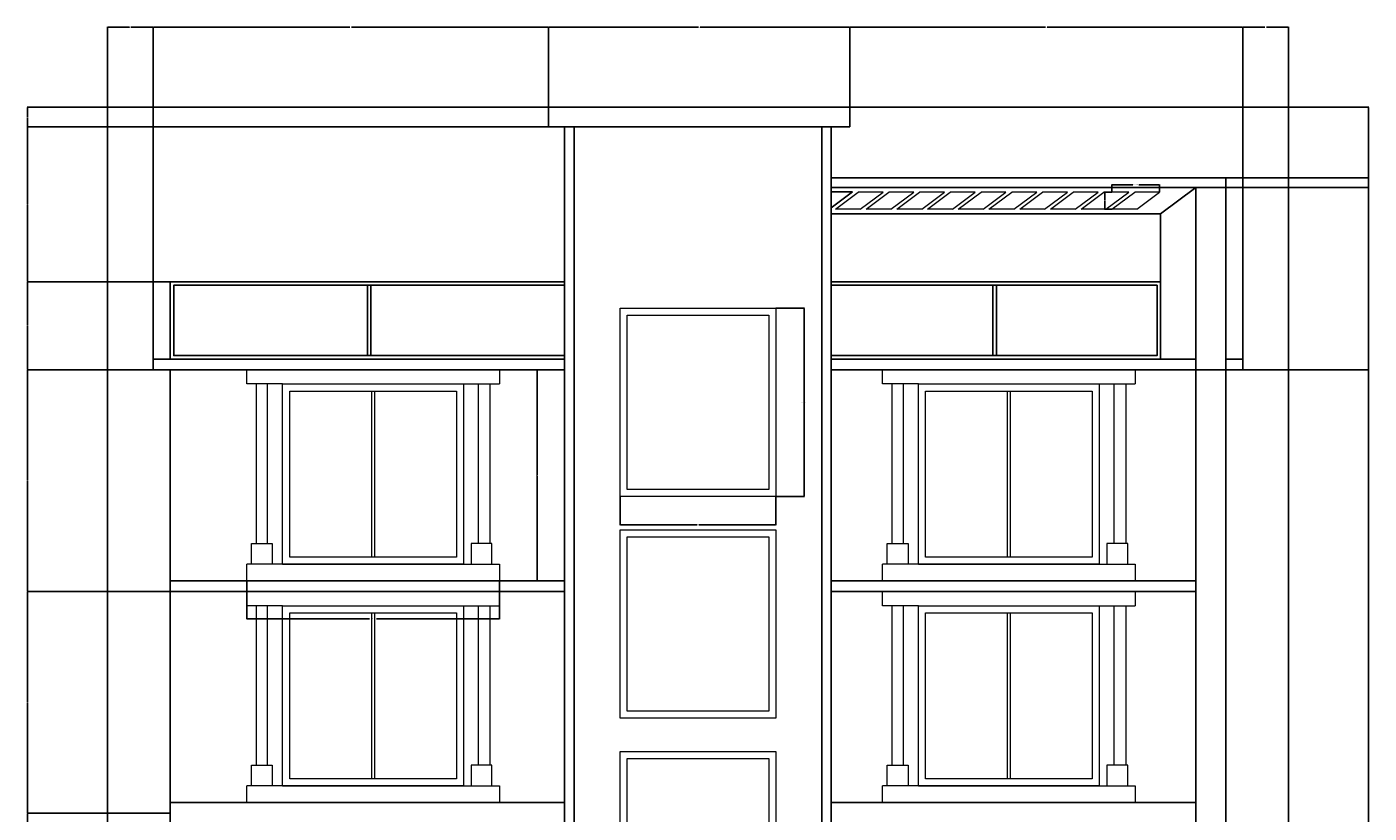
# Model space of a CAD drawing. Units: inches. Extents: x 3024 to 4744, y 1110 to 2100.
# Tile 29 of 29: x 3980 to 4744, y 1654 to 2100. Entities that reach past the tile are written whole.
import ezdxf

# ---------------------------------------------------------------- set-up
doc = ezdxf.new("R2010")
doc.units = ezdxf.units.IN
for name, color, linetype, lineweight in [('A-ANNO-DIMS', 2, 'Continuous', 18), ('A-ELEV', 7, 'Continuous', 25), ('A-GLAZ', 4, 'Continuous', 18), ('A-ROOF', 3, 'Continuous', 18)]:
    doc.layers.add(name, color=color, linetype=linetype, lineweight=lineweight)
doc.styles.get("Standard").update_dxf_attribs({"font": 'arial.ttf'})
doc.dimstyles.get("Standard").update_dxf_attribs({"dimtxt": 0.18, "dimasz": 0.18, "dimexe": 0.18, "dimexo": 0.0625, "dimgap": 0.09, "dimtad": 0, "dimtih": 1, "dimtoh": 1, "dimdec": 1, "dimzin": 0, "dimdsep": 46, "dimlunit": 3, "dimtxsty": 'Standard', "dimcen": 0.09, "dimadec": 0, "dimazin": 0, "dimtfac": 1, "dimtdec": 1, "dimtofl": 0, "dimtmove": 0, "dimatfit": 3, "dimfxl": 1, "dimtolj": 1, "dimtzin": 0, "dimarcsym": 0})

# ---------------------------------------------------------------- blocks, each defined once
blk = doc.blocks.new('WIN-BALCONY-B')
for p, q in [((4125.9, 1897.49), (4105.47, 1897.49)), ((4125.9, 1897.49), (4249.1, 1897.49)), ((4125.9, 1795.04), (4105.47, 1795.04)), ((4125.9, 1795.04), (4249.1, 1795.04))]:
    blk.add_line(p, q)
for points in [[(4105.47, 1897.49), (4105.47, 1905.61), (4249.1, 1905.61), (4249.1, 1897.49)], [(4249.1, 1795.04), (4249.1, 1785.61), (4105.47, 1785.61), (4105.47, 1795.04)]]:
    blk.add_lwpolyline(points)
for points in [[(4110.83, 1806.87), (4117.36, 1806.87), (4117.36, 1897.49), (4110.83, 1897.49)], [(4228.68, 1795.04), (4125.9, 1795.04), (4125.9, 1897.49), (4228.68, 1897.49)], [(4224.68, 1799.04), (4129.9, 1799.04), (4129.9, 1893.49), (4224.68, 1893.49)], [(4176.55, 1893.49), (4178.02, 1893.49), (4178.02, 1799.04), (4176.55, 1799.04)], [(4243.74, 1806.87), (4237.21, 1806.87), (4237.21, 1897.49), (4243.74, 1897.49)], [(4120.03, 1795.04), (4108.16, 1795.04), (4108.16, 1806.87), (4120.03, 1806.87)], [(4233.01, 1795.04), (4244.87, 1795.04), (4244.87, 1806.87), (4233.01, 1806.87)]]:
    blk.add_lwpolyline(points, close=True)
blk = doc.blocks.new('PERGOLA-RAFTER')
for p, q in [((13, 9.73), (0, 0)), ((13, 9.73), (27.14, 9.72)), ((27.14, 9.72), (14.16, 0.01)), ((0, 0), (14.16, 0.01))]:
    blk.add_line(p, q)
blk = doc.blocks.new('WIN-CENTRE-PLAIN')
for points in [[(4317.72, 1940.61), (4406.22, 1940.61), (4406.22, 1833.52), (4317.72, 1833.52)], [(4321.72, 1936.61), (4402.22, 1936.61), (4402.22, 1837.52), (4321.72, 1837.52)]]:
    blk.add_lwpolyline(points, close=True)
blk = doc.blocks.new('*D8')
at = {"layer": 'A-ANNO-DIMS', "color": 0, "lineweight": -2, "transparency": 16777216}
for p, q in [((4105.47, 1785.55), (4105.47, 1763.89)), ((4249.1, 1785.55), (4249.1, 1763.89)), ((4105.65, 1764.07), (4175.35, 1764.07)), ((4248.92, 1764.07), (4179.22, 1764.07))]:
    blk.add_line(p, q, dxfattribs=at)
at = {"layer": 'A-ANNO-DIMS', "color": 0, "transparency": 16777216}
for points in [[(4105.65, 1764.1), (4105.65, 1764.04), (4105.47, 1764.07)], [(4248.92, 1764.1), (4248.92, 1764.04), (4249.1, 1764.07)]]:
    blk.add_solid(points, dxfattribs=at)
at = {"layer": 'Defpoints', "color": 0, "transparency": 16777216}
for p in [(4105.47, 1785.61), (4249.1, 1785.61), (4249.1, 1764.07)]:
    blk.add_point(p, dxfattribs=at)
at = {"layer": 'A-ANNO-DIMS', "color": 0, "transparency": 16777216, "insert": (4177.29, 1764.07), "char_height": 0.18, "attachment_point": 5}
blk.add_mtext('\\A1;BALCONY WINDOW B 144 TYP.', dxfattribs=at)
blk = doc.blocks.new('*D9')
at = {"layer": 'A-ANNO-DIMS', "color": 0, "lineweight": -2, "transparency": 16777216}
for p, q in [((4249.17, 1905.61), (4270.83, 1905.61)), ((4270.65, 1905.43), (4270.65, 1845.79)), ((4270.65, 1785.79), (4270.65, 1845.43)), ((4249.17, 1785.61), (4270.83, 1785.61))]:
    blk.add_line(p, q, dxfattribs=at)
at = {"layer": 'A-ANNO-DIMS', "color": 0, "transparency": 16777216}
for points in [[(4270.62, 1905.43), (4270.68, 1905.43), (4270.65, 1905.61)], [(4270.62, 1785.79), (4270.68, 1785.79), (4270.65, 1785.61)]]:
    blk.add_solid(points, dxfattribs=at)
at = {"layer": 'Defpoints', "color": 0, "transparency": 16777216}
for p in [(4249.1, 1905.61), (4270.65, 1905.61), (4249.1, 1785.61)]:
    blk.add_point(p, dxfattribs=at)
at = {"layer": 'A-ANNO-DIMS', "color": 0, "transparency": 16777216, "insert": (4270.65, 1845.61), "char_height": 0.18, "attachment_point": 5}
blk.add_mtext('\\A1;120 TYP.', dxfattribs=at)
blk = doc.blocks.new('*D12')
at = {"layer": 'A-ANNO-DIMS', "color": 0, "lineweight": -2, "transparency": 16777216}
for p, q in [((4406.28, 1940.61), (4422.46, 1940.61)), ((4422.28, 1940.43), (4422.28, 1887.25)), ((4422.28, 1833.7), (4422.28, 1886.88)), ((4406.28, 1833.52), (4422.46, 1833.52))]:
    blk.add_line(p, q, dxfattribs=at)
at = {"layer": 'A-ANNO-DIMS', "color": 0, "transparency": 16777216}
for points in [[(4422.25, 1940.43), (4422.31, 1940.43), (4422.28, 1940.61)], [(4422.25, 1833.7), (4422.31, 1833.7), (4422.28, 1833.52)]]:
    blk.add_solid(points, dxfattribs=at)
at = {"layer": 'Defpoints', "color": 0, "transparency": 16777216}
for p in [(4406.22, 1940.61), (4422.28, 1940.61), (4406.22, 1833.52)]:
    blk.add_point(p, dxfattribs=at)
at = {"layer": 'A-ANNO-DIMS', "color": 0, "transparency": 16777216, "insert": (4422.28, 1887.07), "char_height": 0.18, "attachment_point": 5}
blk.add_mtext('\\A1;CENTRE WINDOW 107 TYP.', dxfattribs=at)
blk = doc.blocks.new('*D13')
at = {"layer": 'A-ANNO-DIMS', "color": 0, "lineweight": -2, "transparency": 16777216}
for p, q in [((4317.72, 1833.46), (4317.72, 1817.28)), ((4406.22, 1833.46), (4406.22, 1817.28)), ((4317.9, 1817.46), (4361.44, 1817.46)), ((4406.04, 1817.46), (4362.5, 1817.46))]:
    blk.add_line(p, q, dxfattribs=at)
at = {"layer": 'A-ANNO-DIMS', "color": 0, "transparency": 16777216}
for points in [[(4317.9, 1817.49), (4317.9, 1817.43), (4317.72, 1817.46)], [(4406.04, 1817.49), (4406.04, 1817.43), (4406.22, 1817.46)]]:
    blk.add_solid(points, dxfattribs=at)
at = {"layer": 'Defpoints', "color": 0, "transparency": 16777216}
for p in [(4317.72, 1833.52), (4406.22, 1833.52), (4406.22, 1817.46)]:
    blk.add_point(p, dxfattribs=at)
at = {"layer": 'A-ANNO-DIMS', "color": 0, "transparency": 16777216, "insert": (4361.97, 1817.46), "char_height": 0.18, "attachment_point": 5}
blk.add_mtext('\\A1;88 TYP.', dxfattribs=at)
blk = doc.blocks.new('*D14')
at = {"layer": 'A-ANNO-DIMS', "color": 0, "lineweight": -2, "transparency": 16777216}
for p, q in [((4597.25, 2006.58), (4597.25, 2010.77)), ((4597.43, 2010.59), (4609.12, 2010.58)), ((4624.21, 2010.58), (4612.53, 2010.58)), ((4624.39, 2006.57), (4624.39, 2010.76))]:
    blk.add_line(p, q, dxfattribs=at)
at = {"layer": 'A-ANNO-DIMS', "color": 0, "transparency": 16777216}
for points in [[(4597.43, 2010.62), (4597.43, 2010.56), (4597.25, 2010.59)], [(4624.21, 2010.61), (4624.21, 2010.55), (4624.39, 2010.58)]]:
    blk.add_solid(points, dxfattribs=at)
at = {"layer": 'Defpoints', "color": 0, "transparency": 16777216}
for p in [(4597.25, 2010.59), (4597.25, 2006.52), (4624.39, 2006.51)]:
    blk.add_point(p, dxfattribs=at)
at = {"layer": 'A-ANNO-DIMS', "color": 0, "transparency": 16777216, "insert": (4610.82, 2010.58), "char_height": 0.18, "attachment_point": 5}
blk.add_mtext('\\A1;PERGOLA RAFTER 27 TYP.', dxfattribs=at)
blk = doc.blocks.new('*D15')
at = {"layer": 'A-ANNO-DIMS', "color": 0, "lineweight": -2, "transparency": 16777216}
for p, q in [((4597.19, 2006.52), (4593, 2006.52)), ((4593.18, 2006.34), (4593.18, 2001.84)), ((4593.18, 1996.97), (4593.18, 2001.47)), ((4597.18, 1996.79), (4593, 1996.79))]:
    blk.add_line(p, q, dxfattribs=at)
at = {"layer": 'A-ANNO-DIMS', "color": 0, "transparency": 16777216}
for points in [[(4593.15, 2006.34), (4593.21, 2006.34), (4593.18, 2006.52)], [(4593.15, 1996.97), (4593.21, 1996.97), (4593.18, 1996.79)]]:
    blk.add_solid(points, dxfattribs=at)
at = {"layer": 'Defpoints', "color": 0, "transparency": 16777216}
for p in [(4597.25, 2006.52), (4593.18, 1996.79), (4597.25, 1996.79)]:
    blk.add_point(p, dxfattribs=at)
at = {"layer": 'A-ANNO-DIMS', "color": 0, "transparency": 16777216, "insert": (4593.18, 2001.65), "char_height": 0.18, "attachment_point": 5}
blk.add_mtext('\\A1;10 TYP.', dxfattribs=at)
blk = doc.blocks.new('*D30')
at = {"layer": 'A-ANNO-DIMS', "color": 0, "lineweight": -2, "transparency": 16777216}
for p, q in [((4026.29, 1241.5), (4026.29, 2100.44)), ((4026.47, 2100.26), (4038.86, 2100.26)), ((4052.03, 2100.26), (4039.65, 2100.26)), ((4052.21, 1911.67), (4052.21, 2100.44))]:
    blk.add_line(p, q, dxfattribs=at)
at = {"layer": 'A-ANNO-DIMS', "color": 0, "transparency": 16777216}
for points in [[(4026.47, 2100.29), (4026.47, 2100.23), (4026.29, 2100.26)], [(4052.03, 2100.29), (4052.03, 2100.23), (4052.21, 2100.26)]]:
    blk.add_solid(points, dxfattribs=at)
at = {"layer": 'Defpoints', "color": 0, "transparency": 16777216}
for p in [(4052.21, 2100.26), (4052.21, 1911.61), (4026.29, 1241.43)]:
    blk.add_point(p, dxfattribs=at)
at = {"layer": 'A-ANNO-DIMS', "color": 0, "transparency": 16777216, "insert": (4039.25, 2100.26), "char_height": 0.18, "attachment_point": 5}
blk.add_mtext('\\A1;25.92', dxfattribs=at)
blk = doc.blocks.new('*D31')
at = {"layer": 'A-ANNO-DIMS', "color": 0, "lineweight": -2, "transparency": 16777216}
for p, q in [((4052.21, 1911.67), (4052.21, 2100.44)), ((4052.39, 2100.26), (4164.17, 2100.26)), ((4276.88, 2100.26), (4165.11, 2100.26)), ((4277.06, 2054.82), (4277.06, 2100.44))]:
    blk.add_line(p, q, dxfattribs=at)
at = {"layer": 'A-ANNO-DIMS', "color": 0, "transparency": 16777216}
for points in [[(4052.39, 2100.29), (4052.39, 2100.23), (4052.21, 2100.26)], [(4276.88, 2100.29), (4276.88, 2100.23), (4277.06, 2100.26)]]:
    blk.add_solid(points, dxfattribs=at)
at = {"layer": 'Defpoints', "color": 0, "transparency": 16777216}
for p in [(4277.06, 2100.26), (4277.06, 2054.76), (4052.21, 1911.61)]:
    blk.add_point(p, dxfattribs=at)
at = {"layer": 'A-ANNO-DIMS', "color": 0, "transparency": 16777216, "insert": (4164.64, 2100.26), "char_height": 0.18, "attachment_point": 5}
blk.add_mtext('\\A1;224.85', dxfattribs=at)
blk = doc.blocks.new('*D32')
at = {"layer": 'A-ANNO-DIMS', "color": 0, "lineweight": -2, "transparency": 16777216}
for p, q in [((4277.06, 2054.82), (4277.06, 2100.44)), ((4277.24, 2100.26), (4362.24, 2100.26)), ((4448.15, 2100.26), (4363.15, 2100.26)), ((4448.33, 2054.82), (4448.33, 2100.44))]:
    blk.add_line(p, q, dxfattribs=at)
at = {"layer": 'A-ANNO-DIMS', "color": 0, "transparency": 16777216}
for points in [[(4277.24, 2100.29), (4277.24, 2100.23), (4277.06, 2100.26)], [(4448.15, 2100.29), (4448.15, 2100.23), (4448.33, 2100.26)]]:
    blk.add_solid(points, dxfattribs=at)
at = {"layer": 'Defpoints', "color": 0, "transparency": 16777216}
for p in [(4448.33, 2100.26), (4277.06, 2054.76), (4448.33, 2054.76)]:
    blk.add_point(p, dxfattribs=at)
at = {"layer": 'A-ANNO-DIMS', "color": 0, "transparency": 16777216, "insert": (4362.7, 2100.26), "char_height": 0.18, "attachment_point": 5}
blk.add_mtext('\\A1;171.26', dxfattribs=at)
blk = doc.blocks.new('*D33')
at = {"layer": 'A-ANNO-DIMS', "color": 0, "lineweight": -2, "transparency": 16777216}
for p, q in [((4448.33, 2054.82), (4448.33, 2100.44)), ((4448.51, 2100.26), (4559.63, 2100.26)), ((4671.55, 2100.26), (4560.42, 2100.26)), ((4671.73, 1911.67), (4671.73, 2100.44))]:
    blk.add_line(p, q, dxfattribs=at)
at = {"layer": 'A-ANNO-DIMS', "color": 0, "transparency": 16777216}
for points in [[(4448.51, 2100.29), (4448.51, 2100.23), (4448.33, 2100.26)], [(4671.55, 2100.29), (4671.55, 2100.23), (4671.73, 2100.26)]]:
    blk.add_solid(points, dxfattribs=at)
at = {"layer": 'Defpoints', "color": 0, "transparency": 16777216}
for p in [(4671.73, 2100.26), (4448.33, 2054.76), (4671.73, 1911.61)]:
    blk.add_point(p, dxfattribs=at)
at = {"layer": 'A-ANNO-DIMS', "color": 0, "transparency": 16777216, "insert": (4560.03, 2100.26), "char_height": 0.18, "attachment_point": 5}
blk.add_mtext('\\A1;223.4', dxfattribs=at)
blk = doc.blocks.new('*D34')
at = {"layer": 'A-ANNO-DIMS', "color": 0, "lineweight": -2, "transparency": 16777216}
for p, q in [((4671.73, 1911.67), (4671.73, 2100.44)), ((4671.91, 2100.26), (4684.29, 2100.26)), ((4697.47, 2100.26), (4685.08, 2100.26)), ((4697.65, 1241.5), (4697.65, 2100.44))]:
    blk.add_line(p, q, dxfattribs=at)
at = {"layer": 'A-ANNO-DIMS', "color": 0, "transparency": 16777216}
for points in [[(4671.91, 2100.29), (4671.91, 2100.23), (4671.73, 2100.26)], [(4697.47, 2100.29), (4697.47, 2100.23), (4697.65, 2100.26)]]:
    blk.add_solid(points, dxfattribs=at)
at = {"layer": 'Defpoints', "color": 0, "transparency": 16777216}
for p in [(4697.65, 2100.26), (4671.73, 1911.61), (4697.65, 1241.43)]:
    blk.add_point(p, dxfattribs=at)
at = {"layer": 'A-ANNO-DIMS', "color": 0, "transparency": 16777216, "insert": (4684.69, 2100.26), "char_height": 0.18, "attachment_point": 5}
blk.add_mtext('\\A1;25.92', dxfattribs=at)
blk = doc.blocks.new('*D39')
at = {"layer": 'A-ANNO-DIMS', "color": 0, "lineweight": -2, "transparency": 16777216}
for p, q in [((4061.91, 1653.61), (3980.61, 1653.61)), ((3980.79, 1653.43), (3980.79, 1590.79)), ((3980.79, 1527.79), (3980.79, 1590.43)), ((4061.91, 1527.61), (3980.61, 1527.61))]:
    blk.add_line(p, q, dxfattribs=at)
at = {"layer": 'A-ANNO-DIMS', "color": 0, "transparency": 16777216}
for points in [[(3980.76, 1653.43), (3980.82, 1653.43), (3980.79, 1653.61)], [(3980.76, 1527.79), (3980.82, 1527.79), (3980.79, 1527.61)]]:
    blk.add_solid(points, dxfattribs=at)
at = {"layer": 'Defpoints', "color": 0, "transparency": 16777216}
for p in [(3980.79, 1653.61), (4061.97, 1653.61), (4061.97, 1527.61)]:
    blk.add_point(p, dxfattribs=at)
at = {"layer": 'A-ANNO-DIMS', "color": 0, "transparency": 16777216, "insert": (3980.79, 1590.61), "char_height": 0.18, "attachment_point": 5}
blk.add_mtext('\\A1;126', dxfattribs=at)
blk = doc.blocks.new('*D40')
at = {"layer": 'A-ANNO-DIMS', "color": 0, "lineweight": -2, "transparency": 16777216}
for p, q in [((4061.91, 1779.61), (3980.61, 1779.61)), ((3980.79, 1779.43), (3980.79, 1716.79)), ((3980.79, 1653.79), (3980.79, 1716.43)), ((4061.91, 1653.61), (3980.61, 1653.61))]:
    blk.add_line(p, q, dxfattribs=at)
at = {"layer": 'A-ANNO-DIMS', "color": 0, "transparency": 16777216}
for points in [[(3980.76, 1779.43), (3980.82, 1779.43), (3980.79, 1779.61)], [(3980.76, 1653.79), (3980.82, 1653.79), (3980.79, 1653.61)]]:
    blk.add_solid(points, dxfattribs=at)
at = {"layer": 'Defpoints', "color": 0, "transparency": 16777216}
for p in [(3980.79, 1779.61), (4061.97, 1779.61), (4061.97, 1653.61)]:
    blk.add_point(p, dxfattribs=at)
at = {"layer": 'A-ANNO-DIMS', "color": 0, "transparency": 16777216, "insert": (3980.79, 1716.61), "char_height": 0.18, "attachment_point": 5}
blk.add_mtext('\\A1;126', dxfattribs=at)
blk = doc.blocks.new('*D41')
at = {"layer": 'A-ANNO-DIMS', "color": 0, "lineweight": -2, "transparency": 16777216}
for p, q in [((4061.91, 1905.61), (3980.61, 1905.61)), ((3980.79, 1905.43), (3980.79, 1842.79)), ((3980.79, 1779.79), (3980.79, 1842.43)), ((4061.91, 1779.61), (3980.61, 1779.61))]:
    blk.add_line(p, q, dxfattribs=at)
at = {"layer": 'A-ANNO-DIMS', "color": 0, "transparency": 16777216}
for points in [[(3980.76, 1905.43), (3980.82, 1905.43), (3980.79, 1905.61)], [(3980.76, 1779.79), (3980.82, 1779.79), (3980.79, 1779.61)]]:
    blk.add_solid(points, dxfattribs=at)
at = {"layer": 'Defpoints', "color": 0, "transparency": 16777216}
for p in [(3980.79, 1905.61), (4061.97, 1905.61), (4061.97, 1779.61)]:
    blk.add_point(p, dxfattribs=at)
at = {"layer": 'A-ANNO-DIMS', "color": 0, "transparency": 16777216, "insert": (3980.79, 1842.61), "char_height": 0.18, "attachment_point": 5}
blk.add_mtext('\\A1;126', dxfattribs=at)
blk = doc.blocks.new('*D42')
at = {"layer": 'A-ANNO-DIMS', "color": 0, "lineweight": -2, "transparency": 16777216}
for p, q in [((4061.91, 1955.62), (3980.61, 1955.62)), ((3980.79, 1955.44), (3980.79, 1930.8)), ((3980.79, 1905.79), (3980.79, 1930.43)), ((4061.91, 1905.61), (3980.61, 1905.61))]:
    blk.add_line(p, q, dxfattribs=at)
at = {"layer": 'A-ANNO-DIMS', "color": 0, "transparency": 16777216}
for points in [[(3980.76, 1955.44), (3980.82, 1955.44), (3980.79, 1955.62)], [(3980.76, 1905.79), (3980.82, 1905.79), (3980.79, 1905.61)]]:
    blk.add_solid(points, dxfattribs=at)
at = {"layer": 'Defpoints', "color": 0, "transparency": 16777216}
for p in [(3980.79, 1955.62), (4061.97, 1955.62), (4061.97, 1905.61)]:
    blk.add_point(p, dxfattribs=at)
at = {"layer": 'A-ANNO-DIMS', "color": 0, "transparency": 16777216, "insert": (3980.79, 1930.62), "char_height": 0.18, "attachment_point": 5}
blk.add_mtext('\\A1;50.01', dxfattribs=at)
blk = doc.blocks.new('*D43')
at = {"layer": 'A-ANNO-DIMS', "color": 0, "lineweight": -2, "transparency": 16777216}
for p, q in [((4286.14, 2043.53), (3980.61, 2043.53)), ((3980.79, 2043.35), (3980.79, 1999.76)), ((3980.79, 1955.8), (3980.79, 1999.39)), ((4061.91, 1955.62), (3980.61, 1955.62))]:
    blk.add_line(p, q, dxfattribs=at)
at = {"layer": 'A-ANNO-DIMS', "color": 0, "transparency": 16777216}
for points in [[(3980.76, 2043.35), (3980.82, 2043.35), (3980.79, 2043.53)], [(3980.76, 1955.8), (3980.82, 1955.8), (3980.79, 1955.62)]]:
    blk.add_solid(points, dxfattribs=at)
at = {"layer": 'Defpoints', "color": 0, "transparency": 16777216}
for p in [(3980.79, 2043.53), (4286.2, 2043.53), (4061.97, 1955.62)]:
    blk.add_point(p, dxfattribs=at)
at = {"layer": 'A-ANNO-DIMS', "color": 0, "transparency": 16777216, "insert": (3980.79, 1999.57), "char_height": 0.18, "attachment_point": 5}
blk.add_mtext('\\A1;87.91', dxfattribs=at)
blk = doc.blocks.new('*D44')
at = {"layer": 'A-ANNO-DIMS', "color": 0, "lineweight": -2, "transparency": 16777216}
for p, q in [((4277, 2054.76), (3980.61, 2054.76)), ((3980.79, 2054.58), (3980.79, 2049.33)), ((3980.79, 2043.71), (3980.79, 2048.96)), ((4277, 2043.53), (3980.61, 2043.53))]:
    blk.add_line(p, q, dxfattribs=at)
at = {"layer": 'A-ANNO-DIMS', "color": 0, "transparency": 16777216}
for points in [[(3980.76, 2054.58), (3980.82, 2054.58), (3980.79, 2054.76)], [(3980.76, 2043.71), (3980.82, 2043.71), (3980.79, 2043.53)]]:
    blk.add_solid(points, dxfattribs=at)
at = {"layer": 'Defpoints', "color": 0, "transparency": 16777216}
for p in [(3980.79, 2054.76), (4277.06, 2054.76), (4277.06, 2043.53)]:
    blk.add_point(p, dxfattribs=at)
at = {"layer": 'A-ANNO-DIMS', "color": 0, "transparency": 16777216, "insert": (3980.79, 2049.14), "char_height": 0.18, "attachment_point": 5}
blk.add_mtext('\\A1;11.23', dxfattribs=at)
blk = doc.blocks.new('*D48')
at = {"layer": 'A-ANNO-DIMS', "color": 0, "lineweight": -2, "transparency": 16777216}
for p, q in [((4645.12, 2009.17), (4743.33, 2009.17)), ((4743.15, 2008.99), (4743.15, 1957.57)), ((4743.15, 1905.79), (4743.15, 1957.21)), ((4645.12, 1905.61), (4743.33, 1905.61))]:
    blk.add_line(p, q, dxfattribs=at)
at = {"layer": 'A-ANNO-DIMS', "color": 0, "transparency": 16777216}
for points in [[(4743.12, 2008.99), (4743.18, 2008.99), (4743.15, 2009.17)], [(4743.12, 1905.79), (4743.18, 1905.79), (4743.15, 1905.61)]]:
    blk.add_solid(points, dxfattribs=at)
at = {"layer": 'Defpoints', "color": 0, "transparency": 16777216}
for p in [(4645.06, 2009.17), (4743.15, 2009.17), (4645.06, 1905.61)]:
    blk.add_point(p, dxfattribs=at)
at = {"layer": 'A-ANNO-DIMS', "color": 0, "transparency": 16777216, "insert": (4743.15, 1957.39), "char_height": 0.18, "attachment_point": 5}
blk.add_mtext('\\A1;103.56', dxfattribs=at)
blk = doc.blocks.new('*D49')
at = {"layer": 'A-ANNO-DIMS', "color": 0, "lineweight": -2, "transparency": 16777216}
for p, q in [((4662.03, 2014.66), (4743.33, 2014.66)), ((4743.15, 2014.48), (4743.15, 2012.09)), ((4645.12, 2009.17), (4743.33, 2009.17)), ((4743.15, 2009.35), (4743.15, 2011.73))]:
    blk.add_line(p, q, dxfattribs=at)
at = {"layer": 'A-ANNO-DIMS', "color": 0, "transparency": 16777216}
for points in [[(4743.12, 2014.48), (4743.18, 2014.48), (4743.15, 2014.66)], [(4743.12, 2009.35), (4743.18, 2009.35), (4743.15, 2009.17)]]:
    blk.add_solid(points, dxfattribs=at)
at = {"layer": 'Defpoints', "color": 0, "transparency": 16777216}
for p in [(4661.97, 2014.66), (4743.15, 2014.66), (4645.06, 2009.17)]:
    blk.add_point(p, dxfattribs=at)
at = {"layer": 'A-ANNO-DIMS', "color": 0, "transparency": 16777216, "insert": (4743.15, 2011.91), "char_height": 0.18, "attachment_point": 5}
blk.add_mtext('\\A1;5.49', dxfattribs=at)
blk = doc.blocks.new('*D78')
at = {"layer": 'A-ANNO-DIMS', "color": 0, "lineweight": -2, "transparency": 16777216}
for p, q in [((4448.39, 2054.76), (4743.33, 2054.76)), ((4743.15, 2054.58), (4743.15, 1605.37)), ((4743.15, 1155.79), (4743.15, 1605)), ((4697.71, 1155.61), (4743.33, 1155.61))]:
    blk.add_line(p, q, dxfattribs=at)
at = {"layer": 'A-ANNO-DIMS', "color": 0, "transparency": 16777216}
for points in [[(4743.12, 2054.58), (4743.18, 2054.58), (4743.15, 2054.76)], [(4743.12, 1155.79), (4743.18, 1155.79), (4743.15, 1155.61)]]:
    blk.add_solid(points, dxfattribs=at)
at = {"layer": 'Defpoints', "color": 0, "transparency": 16777216}
for p in [(4448.33, 2054.76), (4743.15, 2054.76), (4697.65, 1155.61)]:
    blk.add_point(p, dxfattribs=at)
at = {"layer": 'A-ANNO-DIMS', "color": 0, "transparency": 16777216, "insert": (4743.15, 1605.18), "char_height": 0.18, "attachment_point": 5}
blk.add_mtext('\\A1;899.15', dxfattribs=at)

msp = doc.modelspace()

# ---------------------------------------------------------------- linework, layer by layer
at = {"layer": 'A-ELEV'}
for p, q in [((4645.0576, 2014.6567), (4437.74, 2014.6567)), ((4645.0576, 2009.1664), (4437.74, 2009.1664)), ((4645.0576, 2009.1664), (4624.9779, 1994.1371)), ((4437.74, 2006.6317), (4449.9102, 2006.6233)), ((4449.9102, 2006.6233), (4437.74, 1997.5141)), ((4624.9779, 1994.1371), (4437.74, 1994.1371)), ((4624.9779, 1994.1371), (4624.9779, 1911.6112)), ((4052.2147, 1911.6112), (4286.2022, 1911.6112)), ((4437.74, 1911.6112), (4645.0576, 1911.6112)), ((4661.9711, 1155.6112), (4661.9711, 1911.6112)), ((4061.9711, 1171.0239), (4061.9711, 1905.6112)), ((4286.2022, 1905.6112), (4061.9711, 1905.6112)), ((4645.0576, 1905.6112), (4437.74, 1905.6112)), ((4061.9711, 1785.6112), (4286.2022, 1785.6112)), ((4437.74, 1785.6112), (4645.0576, 1785.6112)), ((4286.2022, 1779.6112), (4061.9711, 1779.6112)), ((4645.0576, 1779.6112), (4437.74, 1779.6112)), ((4061.9711, 1659.6112), (4286.2022, 1659.6112)), ((4437.74, 1659.6112), (4645.0576, 1659.6112))]:
    msp.add_line(p, q, dxfattribs=at)
for points in [[(4448.326, 2043.5286), (4277.0647, 2043.5286), (4277.0647, 2054.7584), (4448.326, 2054.7584)], [(4437.74, 1155.6112), (4286.2022, 1155.6112), (4286.2022, 2043.5286), (4437.74, 2043.5286)], [(4286.2022, 2043.5286), (4291.6033, 2043.5286), (4291.6033, 1155.6112), (4286.2022, 1155.6112)], [(4432.3389, 2043.5286), (4437.74, 2043.5286), (4437.74, 1155.6112), (4432.3389, 1155.6112)]]:
    msp.add_lwpolyline(points, close=True, dxfattribs=at)
for points in [[(4645.0576, 2014.6567), (4661.9711, 2014.6567), (4661.9711, 1905.6112)], [(4661.9711, 1155.6112), (4645.0576, 1155.6112), (4645.0576, 2009.1664)], [(4286.2022, 1955.6193), (4061.9711, 1955.6193), (4061.9711, 1911.6112), (4286.2022, 1911.6112)], [(4286.2022, 1953.6193), (4063.9711, 1953.6193), (4063.9711, 1913.6112), (4286.2022, 1913.6112)], [(4174.0866, 1913.6112), (4174.0866, 1953.6193)], [(4176.0866, 1953.6193), (4176.0866, 1913.6112)], [(4437.74, 1911.6112), (4624.9779, 1911.6112), (4624.9779, 1955.6193), (4437.74, 1955.6193)], [(4437.74, 1913.6112), (4622.9779, 1913.6112), (4622.9779, 1953.6193), (4437.74, 1953.6193)], [(4529.631, 1913.6112), (4529.631, 1953.6193)], [(4531.631, 1953.6193), (4531.631, 1913.6112)], [(4052.2147, 1911.6112), (4052.2147, 1905.6112), (4286.2022, 1905.6112), (4286.2022, 1911.6112)], [(4437.74, 1911.6112), (4437.74, 1905.6112), (4645.0576, 1905.6112)], [(4661.9711, 1905.6112), (4671.7274, 1905.6112), (4671.7274, 1911.6112), (4661.9711, 1911.6112)]]:
    msp.add_lwpolyline(points, dxfattribs=at)

# ---------------------------------------------------------------- block references
at = {"layer": 'A-GLAZ'}
for name, p in [('WIN-CENTRE-PLAIN', (0, 0)), ('WIN-BALCONY-B', (0, 0)), ('WIN-BALCONY-B', (361.4319, 0)), ('WIN-CENTRE-PLAIN', (0, -126)), ('WIN-BALCONY-B', (0, -126)), ('WIN-BALCONY-B', (361.4319, -126)), ('WIN-CENTRE-PLAIN', (0, -252))]:
    msp.add_blockref(name, p, dxfattribs=at)
at = {"layer": 'A-ROOF'}
for p, rotation in [((4467.2095, 2006.5583), 180.1893702113597), ((4484.6741, 2006.5529), 180.1664655150032), ((4502.1386, 2006.5475), 180.1435004991811), ((4519.6032, 2006.542), 180.1204749327306), ((4537.0677, 2006.5366), 180.097388583297), ((4554.5323, 2006.5311), 180.0742412174357), ((4571.9969, 2006.5256), 180.0510326004891), ((4589.4614, 2006.5201), 180.0277624966694), ((4606.926, 2006.5146), 180.0044306689292), ((4624.3906, 2006.5091), 179.9810368794876)]:
    msp.add_blockref('PERGOLA-RAFTER', p, dxfattribs=dict(at, rotation=rotation))

# ---------------------------------------------------------------- dimensions: what is measured, and where the dimension line sits
at = {"layer": 'A-ANNO-DIMS'}
for base, p1, p2, override, picture, middle in [((4052.2147, 2100.2584), (4026.2926, 1241.4341), (4052.2147, 1911.6112), {"dimdec": 2, "dimlfac": 1, "dimrnd": 0, "dimzin": 0, "dimdsep": 46, "dimlunit": 2}, '*D30', (4039.2536, 2100.2584)), ((4277.0647, 2100.2584), (4052.2147, 1911.6112), (4277.0647, 2054.7584), {"dimdec": 2, "dimlfac": 1, "dimrnd": 0, "dimzin": 0, "dimdsep": 46, "dimlunit": 2}, '*D31', (4164.6397, 2100.2584)), ((4448.326, 2100.2584), (4277.0647, 2054.7584), (4448.326, 2054.7584), {"dimdec": 2, "dimlfac": 1, "dimrnd": 0, "dimzin": 0, "dimdsep": 46, "dimlunit": 2}, '*D32', (4362.6954, 2100.2584)), ((4671.7274, 2100.2584), (4448.326, 2054.7584), (4671.7274, 1911.6112), {"dimdec": 1, "dimlfac": 1, "dimrnd": 0, "dimzin": 0, "dimdsep": 46, "dimlunit": 2}, '*D33', (4560.0267, 2100.2584)), ((4697.6496, 2100.2584), (4671.7274, 1911.6112), (4697.6496, 1241.4341), {"dimdec": 2, "dimlfac": 1, "dimrnd": 0, "dimzin": 0, "dimdsep": 46, "dimlunit": 2}, '*D34', (4684.6885, 2100.2584))]:
    dim = msp.add_linear_dim(base=base, p1=p1, p2=p2, dimstyle='Standard', override=override, dxfattribs=at)
    dim.commit()
    dim.dimension.update_dxf_attribs({"geometry": picture, "text_midpoint": middle})
for base, p1, p2, override, picture, middle in [((3980.7926, 2054.7584), (4277.0647, 2043.5286), (4277.0647, 2054.7584), {"dimdec": 2, "dimlfac": 1, "dimrnd": 0, "dimzin": 0, "dimdsep": 46, "dimlunit": 2}, '*D44', (3980.7926, 2049.1435)), ((4743.1496, 2054.7584), (4697.6496, 1155.6112), (4448.326, 2054.7584), {"dimdec": 2, "dimlfac": 1, "dimrnd": 0, "dimzin": 0, "dimdsep": 46, "dimlunit": 2}, '*D78', (4743.1496, 1605.1848)), ((3980.7926, 2043.5286), (4061.9711, 1955.6193), (4286.2022, 2043.5286), {"dimdec": 2, "dimlfac": 1, "dimrnd": 0, "dimzin": 0, "dimdsep": 46, "dimlunit": 2}, '*D43', (3980.7926, 1999.5739)), ((4743.1496, 2014.6567), (4645.0576, 2009.1664), (4661.9711, 2014.6567), {"dimdec": 2, "dimlfac": 1, "dimrnd": 0, "dimzin": 0, "dimdsep": 46, "dimlunit": 2}, '*D49', (4743.1496, 2011.9115)), ((4743.1496, 2009.1664), (4645.0576, 1905.6112), (4645.0576, 2009.1664), {"dimdec": 2, "dimlfac": 1, "dimrnd": 0, "dimzin": 0, "dimdsep": 46, "dimlunit": 2}, '*D48', (4743.1496, 1957.3888)), ((3980.7926, 1955.6193), (4061.9711, 1905.6112), (4061.9711, 1955.6193), {"dimdec": 2, "dimlfac": 1, "dimrnd": 0, "dimzin": 0, "dimdsep": 46, "dimlunit": 2}, '*D42', (3980.7926, 1930.6152)), ((3980.7926, 1905.6112), (4061.9711, 1779.6112), (4061.9711, 1905.6112), {"dimdec": 0, "dimlfac": 1, "dimrnd": 0, "dimzin": 0, "dimdsep": 46, "dimlunit": 2}, '*D41', (3980.7926, 1842.6112)), ((3980.7926, 1779.6112), (4061.9711, 1653.6112), (4061.9711, 1779.6112), {"dimdec": 0, "dimlfac": 1, "dimrnd": 0, "dimzin": 0, "dimdsep": 46, "dimlunit": 2}, '*D40', (3980.7926, 1716.6112)), ((3980.7926, 1653.6112), (4061.9711, 1527.6112), (4061.9711, 1653.6112), {"dimdec": 0, "dimlfac": 1, "dimrnd": 0, "dimzin": 0, "dimdsep": 46, "dimlunit": 2}, '*D39', (3980.7926, 1590.6112))]:
    dim = msp.add_linear_dim(base=base, p1=p1, p2=p2, angle=90, dimstyle='Standard', override=override, dxfattribs=at)
    dim.commit()
    dim.dimension.update_dxf_attribs({"geometry": picture, "text_midpoint": middle})
for base, p1, p2, angle, text, picture, middle in [((4597.2509, 2010.5888), (4624.3905, 2006.5087), (4597.2496, 2006.5177), 179.9810369, 'PERGOLA RAFTER <> TYP.', '*D14', (4610.8214, 2010.5844)), ((4593.1752, 1996.7872), (4597.2496, 2006.5177), (4597.2464, 1996.7858), 269.9810369, '<> TYP.', '*D15', (4593.1768, 2001.6531)), ((4422.2813, 1940.6064), (4406.2191, 1833.5246), (4406.2191, 1940.6064), 90, 'CENTRE WINDOW <> TYP.', '*D12', (4422.2813, 1887.0655)), ((4270.6493, 1905.6112), (4249.104, 1785.6112), (4249.104, 1905.6112), 90, '<> TYP.', '*D9', (4270.6493, 1845.6112))]:
    dim = msp.add_linear_dim(base=base, p1=p1, p2=p2, angle=angle, text=text, dimstyle='Standard', override={"dimdec": 0, "dimrnd": 0, "dimzin": 0, "dimlunit": 2}, dxfattribs=at)
    dim.commit()
    dim.dimension.update_dxf_attribs({"geometry": picture, "text_midpoint": middle})
for base, p1, p2, text, picture, middle in [((4406.2191, 1817.4623), (4317.7231, 1833.5246), (4406.2191, 1833.5246), '<> TYP.', '*D13', (4361.9711, 1817.4623)), ((4249.104, 1764.0658), (4105.4683, 1785.6112), (4249.104, 1785.6112), 'BALCONY WINDOW B <> TYP.', '*D8', (4177.2861, 1764.0658))]:
    dim = msp.add_linear_dim(base=base, p1=p1, p2=p2, text=text, dimstyle='Standard', override={"dimdec": 0, "dimrnd": 0, "dimzin": 0, "dimlunit": 2}, dxfattribs=at)
    dim.commit()
    dim.dimension.update_dxf_attribs({"geometry": picture, "text_midpoint": middle})

doc.saveas('drawing.dxf')
